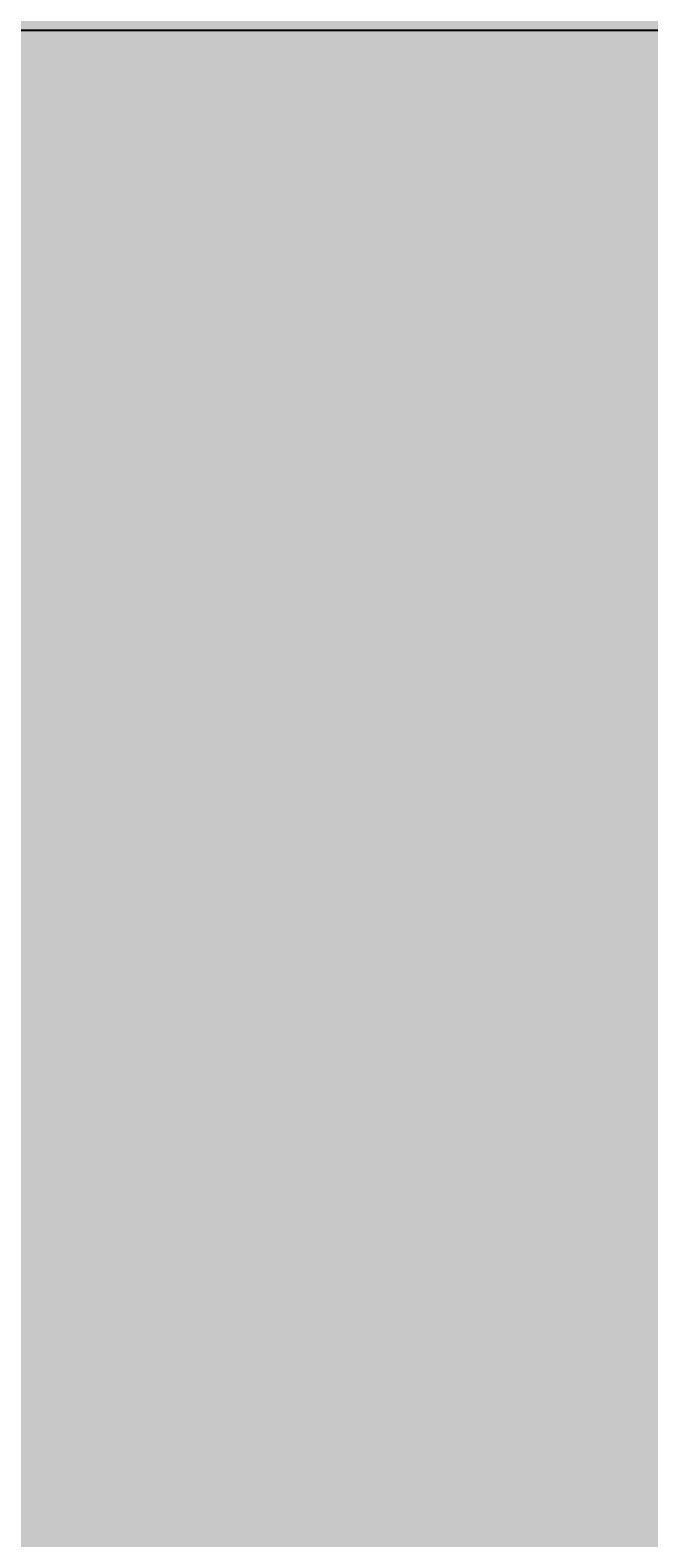
# Model space of a CAD drawing. Units: feet. Extents: x 2695 to 2912, y 795 to 1139.
# Tile 62 of 83: x 2860 to 2877, y 979 to 1021. Entities that reach past the tile are written whole.
import ezdxf

# ---------------------------------------------------------------- set-up
doc = ezdxf.new("R2010")
doc.units = ezdxf.units.FT
doc.layers.add('A-ANNO-DIMS', color=2, linetype='Continuous', lineweight=18)
doc.layers.add('A-ELEV-PATT', color=252, linetype='Continuous', lineweight=13)
doc.styles.get("Standard").update_dxf_attribs({"font": 'arial.ttf'})
doc.dimstyles.get("Standard").update_dxf_attribs({"dimtxt": 0.18, "dimasz": 0.18, "dimexe": 0.18, "dimexo": 0.0625, "dimgap": 0.09, "dimtad": 0, "dimtih": 1, "dimtoh": 1, "dimdec": 1, "dimzin": 0, "dimdsep": 46, "dimlunit": 3, "dimtxsty": 'Standard', "dimcen": 0.09, "dimadec": 0, "dimazin": 0, "dimtfac": 1, "dimtdec": 1, "dimtofl": 0, "dimtmove": 0, "dimatfit": 3, "dimfxl": 1, "dimtolj": 1, "dimtzin": 0, "dimarcsym": 0})

# ---------------------------------------------------------------- blocks, each defined once
blk = doc.blocks.new('*D17')
at = {"layer": 'A-ANNO-DIMS', "color": 0, "lineweight": -2, "transparency": 16777216}
for p, q in [((2843.637, 1020.824), (2911.424, 1020.824)), ((2911.244, 1020.644), (2911.244, 979.059)), ((2911.244, 937.111), (2911.244, 978.695)), ((2890.699, 936.931), (2911.424, 936.931))]:
    blk.add_line(p, q, dxfattribs=at)
at = {"layer": 'A-ANNO-DIMS', "color": 0, "transparency": 16777216}
for points in [[(2911.214, 1020.644), (2911.274, 1020.644), (2911.244, 1020.824)], [(2911.214, 937.111), (2911.274, 937.111), (2911.244, 936.931)]]:
    blk.add_solid(points, dxfattribs=at)
at = {"layer": 'Defpoints', "color": 0, "transparency": 16777216}
for p in [(2843.575, 1020.824), (2911.244, 1020.824), (2890.636, 936.931)]:
    blk.add_point(p, dxfattribs=at)
at = {"layer": 'A-ANNO-DIMS', "color": 0, "transparency": 16777216, "insert": (2911.244, 978.877), "char_height": 0.18, "attachment_point": 5}
blk.add_mtext('\\A1;83.9', dxfattribs=at)
blk = doc.blocks.new('*D50')
at = {"layer": 'A-ANNO-DIMS', "color": 0, "lineweight": -2, "transparency": 16777216}
for p, q in [((2810.041, 972.03), (2810.041, 1138.886)), ((2888.188, 972.03), (2888.188, 1138.886)), ((2810.221, 1138.706), (2848.721, 1138.706)), ((2888.008, 1138.706), (2849.508, 1138.706))]:
    blk.add_line(p, q, dxfattribs=at)
at = {"layer": 'A-ANNO-DIMS', "color": 0, "transparency": 16777216}
for points in [[(2810.221, 1138.736), (2810.221, 1138.676), (2810.041, 1138.706)], [(2888.008, 1138.736), (2888.008, 1138.676), (2888.188, 1138.706)]]:
    blk.add_solid(points, dxfattribs=at)
at = {"layer": 'Defpoints', "color": 0, "transparency": 16777216}
for p in [(2888.188, 1138.706), (2810.041, 971.967), (2888.188, 971.967)]:
    blk.add_point(p, dxfattribs=at)
at = {"layer": 'A-ANNO-DIMS', "color": 0, "transparency": 16777216, "insert": (2849.114, 1138.706), "char_height": 0.18, "attachment_point": 5}
blk.add_mtext('\\A1;78.15', dxfattribs=at)

msp = doc.modelspace()

# ---------------------------------------------------------------- hatches: boundary and pattern name
at = {"layer": 'A-ELEV-PATT'}
h = msp.add_hatch(color=256, dxfattribs=at)
h.set_gradient(color1=(147, 149, 152), color2=(147, 149, 152), tint=1)
h.paths.add_polyline_path([(2770.6361, 1118.4096), (2710.6361, 1118.4096), (2710.6361, 1062.9306), (2770.6361, 1062.9306)])
h.paths.add_polyline_path([(2890.6361, 1103.3378), (2770.6361, 1103.3378), (2770.6361, 1062.9306), (2890.6361, 1062.9306)])
h.paths.add_polyline_path([(2730.7081, 1048.1052), (2755.1125, 1048.1052), (2755.1125, 936.9306), (2770.6361, 936.9306), (2770.6361, 1050.3105), (2715.8852, 1050.3105), (2715.8852, 936.9306), (2730.7081, 936.9306)])
h.paths.add_polyline_path([(2890.6361, 1050.3105), (2770.6361, 1050.3105), (2770.6361, 971.9673), (2778.0341, 971.9673), (2778.0341, 1020.8235), (2843.575, 1020.8235), (2843.575, 971.9673), (2890.6361, 971.9673)])
h.paths.add_polyline_path([(2888.1882, 970.7156), (2843.575, 970.7156), (2843.575, 964.8267), (2888.1882, 964.8267)])
h.paths.add_polyline_path([(2888.1882, 964.1328), (2843.575, 964.1328), (2843.575, 956.614), (2888.1882, 956.614)])
h.paths.add_polyline_path([(2888.1882, 955.9202), (2843.575, 955.9202), (2843.575, 949.2892), (2888.1882, 949.2892)])
h.paths.add_polyline_path([(2888.1882, 948.5954), (2843.575, 948.5954), (2843.575, 941.3507), (2888.1882, 941.3507)])
h.paths.add_polyline_path([(2888.1882, 940.6569), (2843.575, 940.6569), (2843.575, 936.9306), (2888.1882, 936.9306)])
h.paths.add_polyline_path([(2890.6361, 970.7156), (2888.9368, 970.7156), (2888.9368, 964.8267), (2890.6361, 964.8267)])
h.paths.add_polyline_path([(2890.6361, 964.1328), (2888.9368, 964.1328), (2888.9368, 956.614), (2890.6361, 956.614)])
h.paths.add_polyline_path([(2890.6361, 955.9202), (2888.9368, 955.9202), (2888.9368, 949.2892), (2890.6361, 949.2892)])
h.paths.add_polyline_path([(2890.6361, 940.6569), (2888.9368, 940.6569), (2888.9368, 936.9306), (2890.6361, 936.9306)])
h.paths.add_polyline_path([(2890.6361, 948.5954), (2888.9368, 948.5954), (2888.9368, 941.3507), (2890.6361, 941.3507)])
h.paths.add_polyline_path([(2772.5216, 970.7156), (2770.6361, 970.7156), (2770.6361, 964.8267), (2772.5216, 964.8267)])
h.paths.add_polyline_path([(2772.5216, 964.1328), (2770.6361, 964.1328), (2770.6361, 956.614), (2772.5216, 956.614)])
h.paths.add_polyline_path([(2772.5216, 955.9202), (2770.6361, 955.9202), (2770.6361, 949.2892), (2772.5216, 949.2892)])
h.paths.add_polyline_path([(2772.5216, 948.5954), (2770.6361, 948.5954), (2770.6361, 941.3507), (2772.5216, 941.3507)])
h.paths.add_polyline_path([(2772.5216, 940.6569), (2770.6361, 940.6569), (2770.6361, 936.9306), (2772.5216, 936.9306)])
h.paths.add_polyline_path([(2778.0341, 940.6569), (2773.2702, 940.6569), (2773.2702, 936.9306), (2778.0341, 936.9306)])
h.paths.add_polyline_path([(2778.0341, 970.7156), (2773.2702, 970.7156), (2773.2702, 964.8267), (2778.0341, 964.8267)])
h.paths.add_polyline_path([(2778.0341, 964.1328), (2773.2702, 964.1328), (2773.2702, 956.614), (2778.0341, 956.614)])
h.paths.add_polyline_path([(2778.0341, 955.9202), (2773.2702, 955.9202), (2773.2702, 949.2892), (2778.0341, 949.2892)])
h.paths.add_polyline_path([(2778.0341, 948.5954), (2773.2702, 948.5954), (2773.2702, 941.3507), (2778.0341, 941.3507)])
h.paths.add_polyline_path([(2810.0407, 940.6569), (2780.0341, 940.6569), (2780.0341, 936.9306), (2810.0407, 936.9306)])
h.paths.add_polyline_path([(2890.6361, 924.3105), (2770.6361, 924.3105), (2770.6361, 810.9306), (2773.5029, 810.9306), (2773.5029, 905.5143), (2805.9398, 905.5143), (2838.3767, 905.5143), (2838.3767, 810.9306), (2890.6361, 810.9306)])

# ---------------------------------------------------------------- dimensions: what is measured, and where the dimension line sits
at = {"layer": 'A-ANNO-DIMS'}
dim = msp.add_linear_dim(base=(2888.1882, 1138.7056), p1=(2810.0407, 971.9673), p2=(2888.1882, 971.9673), dimstyle='Standard', override={"dimdec": 2, "dimlfac": 1, "dimrnd": 0, "dimzin": 0, "dimdsep": 46, "dimlunit": 2}, dxfattribs=at)
dim.commit()
dim.dimension.update_dxf_attribs({"geometry": '*D50', "text_midpoint": (2849.1144, 1138.7056)})
dim = msp.add_linear_dim(base=(2911.2444, 1020.8235), p1=(2890.6361, 936.9306), p2=(2843.575, 1020.8235), angle=90, dimstyle='Standard', override={"dimdec": 1, "dimlfac": 1, "dimrnd": 0, "dimzin": 0, "dimdsep": 46, "dimlunit": 2}, dxfattribs=at)
dim.commit()
dim.dimension.update_dxf_attribs({"geometry": '*D17', "text_midpoint": (2911.2444, 978.877)})

doc.saveas('drawing.dxf')
